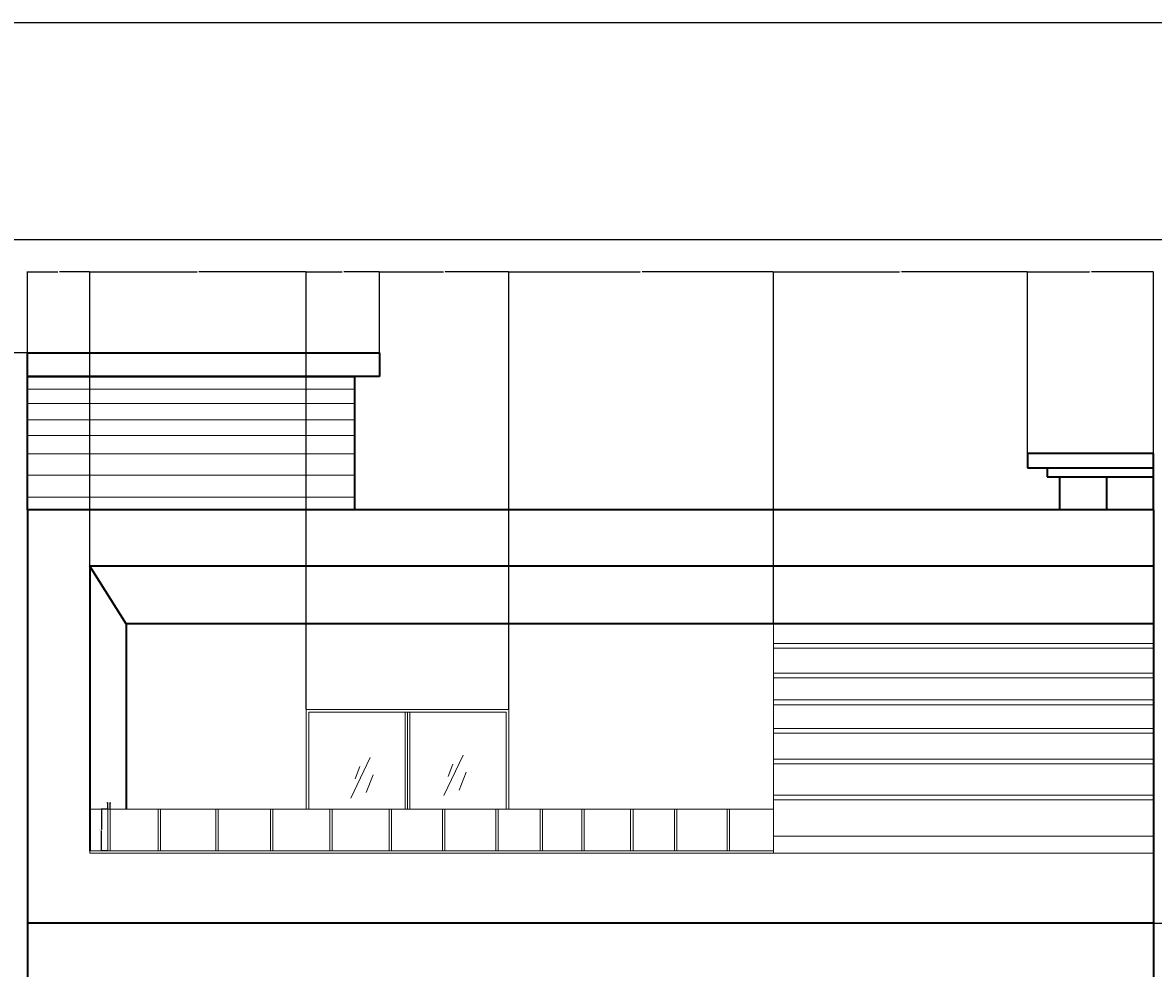
# Model space of a CAD drawing. Units: inches. Extents: x 1770 to 2988, y 1161 to 3221.
# Tile 36 of 44: x 2179 to 2655, y 2823 to 3221. Entities that reach past the tile are written whole.
import ezdxf

# ---------------------------------------------------------------- set-up
doc = ezdxf.new("R2010")
doc.units = ezdxf.units.IN
for name, color, linetype, lineweight in [('A-ANNO-DIMS', 2, 'Continuous', 18), ('A-ANNO-TTLB', 7, 'Continuous', 25), ('A-ELEV', 7, 'Continuous', 35), ('A-ELEV-DETL', 7, 'Continuous', 18), ('A-ELEV-GLAZ', 4, 'Continuous', 18)]:
    doc.layers.add(name, color=color, linetype=linetype, lineweight=lineweight)
doc.styles.get("Standard").update_dxf_attribs({"font": 'arial.ttf'})
doc.dimstyles.get("Standard").update_dxf_attribs({"dimtxt": 0.18, "dimasz": 0.18, "dimexe": 0.18, "dimexo": 0.0625, "dimgap": 0.09, "dimtad": 0, "dimtih": 1, "dimtoh": 1, "dimdec": 4, "dimzin": 0, "dimdsep": 46, "dimtxsty": 'Standard', "dimcen": 0.09, "dimadec": 0, "dimazin": 0, "dimtfac": 1, "dimtdec": 4, "dimtofl": 0, "dimtmove": 0, "dimatfit": 3, "dimfxl": 1, "dimtolj": 1, "dimtzin": 0, "dimarcsym": 0})

# ---------------------------------------------------------------- blocks, each defined once
blk = doc.blocks.new('GLASS-MARK-UPPER')
for p, q in [((8.2, 17.02), (0, 0)), ((3.76, 13.29), (1.82, 8.07)), ((9.37, 9.81), (6.4, 2.34))]:
    blk.add_line(p, q)
blk = doc.blocks.new('BALCONY-BALUSTER-ELEV')
for p, q in [((0, 17.5), (0, 0)), ((1, 0), (1, 17.5))]:
    blk.add_line(p, q)
blk = doc.blocks.new('*D54')
at = {"layer": 'A-ANNO-DIMS', "color": 0, "lineweight": -2, "transparency": 16777216}
for p, q in [((2215.14, 2890.3), (2212.39, 2890.3)), ((2212.57, 2890.12), (2212.57, 2881.73)), ((2212.57, 2872.97), (2212.57, 2881.36)), ((2215.14, 2872.79), (2212.39, 2872.79))]:
    blk.add_line(p, q, dxfattribs=at)
at = {"layer": 'A-ANNO-DIMS', "color": 0, "transparency": 16777216}
for points in [[(2212.54, 2890.12), (2212.6, 2890.12), (2212.57, 2890.3)], [(2212.54, 2872.97), (2212.6, 2872.97), (2212.57, 2872.79)]]:
    blk.add_solid(points, dxfattribs=at)
at = {"layer": 'Defpoints', "color": 0, "transparency": 16777216}
for p in [(2212.57, 2890.3), (2215.2, 2890.3), (2215.2, 2872.79)]:
    blk.add_point(p, dxfattribs=at)
at = {"layer": 'A-ANNO-DIMS', "color": 0, "transparency": 16777216, "insert": (2212.57, 2881.55), "char_height": 0.18, "attachment_point": 5}
blk.add_mtext('\\A1;BALUSTER 18 TYP.', dxfattribs=at)
blk = doc.blocks.new('*D55')
at = {"layer": 'A-ANNO-DIMS', "color": 0, "lineweight": -2, "transparency": 16777216}
for p, q in [((2215.02, 2892.92), (2214.84, 2892.92)), ((2215.2, 2890.36), (2215.2, 2893.1)), ((2216.2, 2890.36), (2216.2, 2893.1)), ((2216.38, 2892.92), (2216.56, 2892.92))]:
    blk.add_line(p, q, dxfattribs=at)
at = {"layer": 'A-ANNO-DIMS', "color": 0, "transparency": 16777216}
for points in [[(2215.02, 2892.95), (2215.02, 2892.89), (2215.2, 2892.92)], [(2216.38, 2892.95), (2216.38, 2892.89), (2216.2, 2892.92)]]:
    blk.add_solid(points, dxfattribs=at)
at = {"layer": 'Defpoints', "color": 0, "transparency": 16777216}
for p in [(2215.2, 2890.3), (2216.2, 2892.92), (2216.2, 2890.3)]:
    blk.add_point(p, dxfattribs=at)
at = {"layer": 'A-ANNO-DIMS', "color": 0, "transparency": 16777216, "insert": (2215.7, 2892.92), "char_height": 0.18, "attachment_point": 5}
blk.add_mtext('\\A1;1 TYP.', dxfattribs=at)
blk = doc.blocks.new('*D94')
at = {"layer": 'A-ANNO-DIMS', "color": 0, "lineweight": -2, "transparency": 16777216}
for p, q in [((2181.38, 3082.38), (2059.85, 3082.38)), ((2060.03, 3082.2), (2060.03, 2893.52)), ((2060.03, 2704.48), (2060.03, 2893.16)), ((2181.38, 2704.3), (2059.85, 2704.3))]:
    blk.add_line(p, q, dxfattribs=at)
at = {"layer": 'A-ANNO-DIMS', "color": 0, "transparency": 16777216}
for points in [[(2060, 3082.2), (2060.06, 3082.2), (2060.03, 3082.38)], [(2060, 2704.48), (2060.06, 2704.48), (2060.03, 2704.3)]]:
    blk.add_solid(points, dxfattribs=at)
at = {"layer": 'Defpoints', "color": 0, "transparency": 16777216}
for p in [(2060.03, 3082.38), (2181.44, 3082.38), (2181.44, 2704.3)]:
    blk.add_point(p, dxfattribs=at)
at = {"layer": 'A-ANNO-DIMS', "color": 0, "transparency": 16777216, "insert": (2060.03, 2893.34), "char_height": 0.18, "attachment_point": 5}
blk.add_mtext('\\A1;378.1', dxfattribs=at)
blk = doc.blocks.new('*D98')
at = {"layer": 'A-ANNO-DIMS', "color": 0, "lineweight": -2, "transparency": 16777216}
for p, q in [((2655.51, 2842.3), (2801.91, 2842.3)), ((2801.73, 2842.12), (2801.73, 2824.48)), ((2801.73, 2806.48), (2801.73, 2824.11)), ((2620.11, 2806.3), (2801.91, 2806.3))]:
    blk.add_line(p, q, dxfattribs=at)
at = {"layer": 'A-ANNO-DIMS', "color": 0, "transparency": 16777216}
for points in [[(2801.7, 2842.12), (2801.76, 2842.12), (2801.73, 2842.3)], [(2801.7, 2806.48), (2801.76, 2806.48), (2801.73, 2806.3)]]:
    blk.add_solid(points, dxfattribs=at)
at = {"layer": 'Defpoints', "color": 0, "transparency": 16777216}
for p in [(2655.44, 2842.3), (2801.73, 2842.3), (2620.05, 2806.3)]:
    blk.add_point(p, dxfattribs=at)
at = {"layer": 'A-ANNO-DIMS', "color": 0, "transparency": 16777216, "insert": (2801.73, 2824.3), "char_height": 0.18, "attachment_point": 5}
blk.add_mtext('\\A1;36', dxfattribs=at)
blk = doc.blocks.new('*D103')
at = {"layer": 'A-ANNO-DIMS', "color": 0, "lineweight": -2, "transparency": 16777216}
for p, q in [((2181.44, 3082.44), (2181.44, 3116.56)), ((2181.62, 3116.38), (2194.16, 3116.38)), ((2207.49, 3116.38), (2194.95, 3116.38)), ((2207.67, 2992.61), (2207.67, 3116.56))]:
    blk.add_line(p, q, dxfattribs=at)
at = {"layer": 'A-ANNO-DIMS', "color": 0, "transparency": 16777216}
for points in [[(2181.62, 3116.41), (2181.62, 3116.35), (2181.44, 3116.38)], [(2207.49, 3116.41), (2207.49, 3116.35), (2207.67, 3116.38)]]:
    blk.add_solid(points, dxfattribs=at)
at = {"layer": 'Defpoints', "color": 0, "transparency": 16777216}
for p in [(2207.67, 3116.38), (2181.44, 3082.38), (2207.67, 2992.55)]:
    blk.add_point(p, dxfattribs=at)
at = {"layer": 'A-ANNO-DIMS', "color": 0, "transparency": 16777216, "insert": (2194.56, 3116.38), "char_height": 0.18, "attachment_point": 5}
blk.add_mtext('\\A1;26.23', dxfattribs=at)
blk = doc.blocks.new('*D104')
at = {"layer": 'A-ANNO-DIMS', "color": 0, "lineweight": -2, "transparency": 16777216}
for p, q in [((2207.67, 2992.61), (2207.67, 3116.56)), ((2207.85, 3116.38), (2252.84, 3116.38)), ((2298.61, 3116.38), (2253.62, 3116.38)), ((2298.79, 2932.36), (2298.79, 3116.56))]:
    blk.add_line(p, q, dxfattribs=at)
at = {"layer": 'A-ANNO-DIMS', "color": 0, "transparency": 16777216}
for points in [[(2207.85, 3116.41), (2207.85, 3116.35), (2207.67, 3116.38)], [(2298.61, 3116.41), (2298.61, 3116.35), (2298.79, 3116.38)]]:
    blk.add_solid(points, dxfattribs=at)
at = {"layer": 'Defpoints', "color": 0, "transparency": 16777216}
for p in [(2298.79, 3116.38), (2207.67, 2992.55), (2298.79, 2932.3)]:
    blk.add_point(p, dxfattribs=at)
at = {"layer": 'A-ANNO-DIMS', "color": 0, "transparency": 16777216, "insert": (2253.23, 3116.38), "char_height": 0.18, "attachment_point": 5}
blk.add_mtext('\\A1;91.12', dxfattribs=at)
blk = doc.blocks.new('*D105')
at = {"layer": 'A-ANNO-DIMS', "color": 0, "lineweight": -2, "transparency": 16777216}
for p, q in [((2298.79, 2932.36), (2298.79, 3116.56)), ((2298.97, 3116.38), (2313.84, 3116.38)), ((2329.5, 3116.38), (2314.63, 3116.38)), ((2329.68, 3082.44), (2329.68, 3116.56))]:
    blk.add_line(p, q, dxfattribs=at)
at = {"layer": 'A-ANNO-DIMS', "color": 0, "transparency": 16777216}
for points in [[(2298.97, 3116.41), (2298.97, 3116.35), (2298.79, 3116.38)], [(2329.5, 3116.41), (2329.5, 3116.35), (2329.68, 3116.38)]]:
    blk.add_solid(points, dxfattribs=at)
at = {"layer": 'Defpoints', "color": 0, "transparency": 16777216}
for p in [(2329.68, 3116.38), (2329.68, 3082.38), (2298.79, 2932.3)]:
    blk.add_point(p, dxfattribs=at)
at = {"layer": 'A-ANNO-DIMS', "color": 0, "transparency": 16777216, "insert": (2314.23, 3116.38), "char_height": 0.18, "attachment_point": 5}
blk.add_mtext('\\A1;30.89', dxfattribs=at)
blk = doc.blocks.new('*D106')
at = {"layer": 'A-ANNO-DIMS', "color": 0, "lineweight": -2, "transparency": 16777216}
for p, q in [((2329.68, 3082.44), (2329.68, 3116.56)), ((2329.86, 3116.38), (2356.51, 3116.38)), ((2383.95, 3116.38), (2357.3, 3116.38)), ((2384.13, 2932.36), (2384.13, 3116.56))]:
    blk.add_line(p, q, dxfattribs=at)
at = {"layer": 'A-ANNO-DIMS', "color": 0, "transparency": 16777216}
for points in [[(2329.86, 3116.41), (2329.86, 3116.35), (2329.68, 3116.38)], [(2383.95, 3116.41), (2383.95, 3116.35), (2384.13, 3116.38)]]:
    blk.add_solid(points, dxfattribs=at)
at = {"layer": 'Defpoints', "color": 0, "transparency": 16777216}
for p in [(2384.13, 3116.38), (2329.68, 3082.38), (2384.13, 2932.3)]:
    blk.add_point(p, dxfattribs=at)
at = {"layer": 'A-ANNO-DIMS', "color": 0, "transparency": 16777216, "insert": (2356.91, 3116.38), "char_height": 0.18, "attachment_point": 5}
blk.add_mtext('\\A1;54.46', dxfattribs=at)
blk = doc.blocks.new('*D107')
at = {"layer": 'A-ANNO-DIMS', "color": 0, "lineweight": -2, "transparency": 16777216}
for p, q in [((2384.13, 2932.36), (2384.13, 3116.56)), ((2384.31, 3116.38), (2439.34, 3116.38)), ((2495.29, 3116.38), (2440.25, 3116.38)), ((2495.47, 2968.36), (2495.47, 3116.56))]:
    blk.add_line(p, q, dxfattribs=at)
at = {"layer": 'A-ANNO-DIMS', "color": 0, "transparency": 16777216}
for points in [[(2384.31, 3116.41), (2384.31, 3116.35), (2384.13, 3116.38)], [(2495.29, 3116.41), (2495.29, 3116.35), (2495.47, 3116.38)]]:
    blk.add_solid(points, dxfattribs=at)
at = {"layer": 'Defpoints', "color": 0, "transparency": 16777216}
for p in [(2495.47, 3116.38), (2495.47, 2968.3), (2384.13, 2932.3)]:
    blk.add_point(p, dxfattribs=at)
at = {"layer": 'A-ANNO-DIMS', "color": 0, "transparency": 16777216, "insert": (2439.8, 3116.38), "char_height": 0.18, "attachment_point": 5}
blk.add_mtext('\\A1;111.33', dxfattribs=at)
blk = doc.blocks.new('*D108')
at = {"layer": 'A-ANNO-DIMS', "color": 0, "lineweight": -2, "transparency": 16777216}
for p, q in [((2495.47, 2968.36), (2495.47, 3116.56)), ((2495.65, 3116.38), (2548.52, 3116.38)), ((2602.31, 3116.38), (2549.43, 3116.38)), ((2602.49, 3040.08), (2602.49, 3116.56))]:
    blk.add_line(p, q, dxfattribs=at)
at = {"layer": 'A-ANNO-DIMS', "color": 0, "transparency": 16777216}
for points in [[(2495.65, 3116.41), (2495.65, 3116.35), (2495.47, 3116.38)], [(2602.31, 3116.41), (2602.31, 3116.35), (2602.49, 3116.38)]]:
    blk.add_solid(points, dxfattribs=at)
at = {"layer": 'Defpoints', "color": 0, "transparency": 16777216}
for p in [(2602.49, 3116.38), (2602.49, 3040.02), (2495.47, 2968.3)]:
    blk.add_point(p, dxfattribs=at)
at = {"layer": 'A-ANNO-DIMS', "color": 0, "transparency": 16777216, "insert": (2548.98, 3116.38), "char_height": 0.18, "attachment_point": 5}
blk.add_mtext('\\A1;107.02', dxfattribs=at)
blk = doc.blocks.new('*D109')
at = {"layer": 'A-ANNO-DIMS', "color": 0, "lineweight": -2, "transparency": 16777216}
for p, q in [((2602.49, 3040.08), (2602.49, 3116.56)), ((2602.67, 3116.38), (2628.57, 3116.38)), ((2655.26, 3116.38), (2629.36, 3116.38)), ((2655.44, 3040.08), (2655.44, 3116.56))]:
    blk.add_line(p, q, dxfattribs=at)
at = {"layer": 'A-ANNO-DIMS', "color": 0, "transparency": 16777216}
for points in [[(2602.67, 3116.41), (2602.67, 3116.35), (2602.49, 3116.38)], [(2655.26, 3116.41), (2655.26, 3116.35), (2655.44, 3116.38)]]:
    blk.add_solid(points, dxfattribs=at)
at = {"layer": 'Defpoints', "color": 0, "transparency": 16777216}
for p in [(2655.44, 3116.38), (2602.49, 3040.02), (2655.44, 3040.02)]:
    blk.add_point(p, dxfattribs=at)
at = {"layer": 'A-ANNO-DIMS', "color": 0, "transparency": 16777216, "insert": (2628.96, 3116.38), "char_height": 0.18, "attachment_point": 5}
blk.add_mtext('\\A1;52.96', dxfattribs=at)

msp = doc.modelspace()

# ---------------------------------------------------------------- linework, layer by layer
at = {"layer": 'A-ANNO-TTLB'}
for points in [[(1769.9155, 3221.2788), (2987.7567, 3221.2788), (2987.7567, 1161.1516), (1769.9155, 1161.1516)], [(2073.6202, 3129.9468), (2769.3644, 3129.9468), (2769.3644, 2546.8952), (2073.6202, 2546.8952)]]:
    msp.add_lwpolyline(points, close=True, dxfattribs=at)
at = {"layer": 'A-ELEV'}
for p, q in [((2181.443, 3016.2969), (2181.443, 3082.3817)), ((2181.443, 3082.3817), (2329.6779, 3082.3817)), ((2329.6779, 3082.3817), (2329.6779, 3072.4167)), ((2329.6779, 3072.4167), (2181.443, 3072.4167)), ((2181.443, 3072.4167), (2319.1337, 3072.4167)), ((2319.1337, 3072.4167), (2319.1337, 3016.2969)), ((2655.443, 3040.0203), (2602.4869, 3040.0203)), ((2602.4869, 3040.0203), (2602.4869, 3033.8964)), ((2655.443, 3016.2969), (2655.443, 3040.0203)), ((2602.4869, 3033.8964), (2610.7495, 3033.8964)), ((2610.7495, 3033.8964), (2610.7495, 3030.156)), ((2610.7495, 3033.8964), (2655.443, 3033.8964)), ((2655.443, 3033.8964), (2655.443, 3033.8964)), ((2610.7495, 3030.156), (2615.954, 3030.156)), ((2615.954, 3030.156), (2615.954, 3016.2969)), ((2615.954, 3030.156), (2655.443, 3030.156)), ((2635.6985, 3030.156), (2635.6985, 3016.2969)), ((2181.443, 3016.2969), (2181.443, 2830.2969)), ((2655.443, 3016.2969), (2181.443, 3016.2969)), ((2655.443, 3016.2969), (2655.443, 2830.2969)), ((2655.443, 2992.5451), (2207.6717, 2992.5451)), ((2207.6717, 2992.5451), (2207.6717, 2872.7943)), ((2223.0291, 2968.2969), (2207.6717, 2992.5451)), ((2655.443, 2968.2969), (2223.0291, 2968.2969)), ((2223.0291, 2968.2969), (2223.0291, 2890.2969)), ((2181.443, 2890.2969), (2181.443, 2704.2969)), ((2655.443, 2890.2969), (2655.443, 2704.2969)), ((2655.443, 2842.2969), (2181.443, 2842.2969))]:
    msp.add_line(p, q, dxfattribs=at)
at = {"layer": 'A-ELEV-DETL'}
for p, q in [((2181.443, 3067.0892), (2319.1337, 3067.0892)), ((2181.443, 3061.03), (2319.1337, 3061.03)), ((2181.443, 3054.1618), (2319.1337, 3054.1618)), ((2181.443, 3047.5875), (2319.1337, 3047.5875)), ((2181.443, 3039.8117), (2319.1337, 3039.8117)), ((2181.443, 3030.8799), (2319.1337, 3030.8799)), ((2181.443, 3021.5728), (2319.1337, 3021.5728)), ((2495.4654, 2871.7943), (2495.4654, 2968.2969)), ((2495.4654, 2960.0436), (2655.443, 2960.0436)), ((2655.443, 2958.0436), (2495.4654, 2958.0436)), ((2655.443, 2960.0436), (2655.443, 2958.0436)), ((2495.4654, 2947.5038), (2655.443, 2947.5038)), ((2655.443, 2945.5038), (2495.4654, 2945.5038)), ((2495.4654, 2936.259), (2655.443, 2936.259)), ((2655.443, 2934.259), (2495.4654, 2934.259)), ((2495.4654, 2924.2391), (2655.443, 2924.2391)), ((2655.443, 2922.2391), (2495.4654, 2922.2391)), ((2495.4654, 2911.3321), (2655.443, 2911.3321)), ((2655.443, 2909.3321), (2495.4654, 2909.3321)), ((2495.4654, 2896.1676), (2655.443, 2896.1676)), ((2444.1544, 2890.2969), (2207.6717, 2890.2969)), ((2236.4714, 2890.2969), (2236.4714, 2872.7943)), ((2237.4714, 2872.7943), (2237.4714, 2890.2969)), ((2414.828, 2890.2969), (2414.828, 2872.7943)), ((2414.828, 2890.2969), (2414.828, 2872.7943)), ((2415.828, 2872.7943), (2415.828, 2890.2969)), ((2415.828, 2872.7943), (2415.828, 2890.2969)), ((2444.1544, 2890.2969), (2495.4654, 2890.2969)), ((2655.443, 2894.1676), (2495.4654, 2894.1676)), ((2655.443, 2872.7943), (2655.443, 2885.1589)), ((2655.443, 2878.9766), (2495.4654, 2878.9766)), ((2655.443, 2871.7943), (2655.443, 2878.9766)), ((2207.6717, 2872.7943), (2444.1544, 2872.7943)), ((2207.6717, 2872.7943), (2207.6717, 2871.7943)), ((2207.6717, 2871.7943), (2444.1544, 2871.7943)), ((2236.4714, 2872.7943), (2237.4714, 2872.7943)), ((2444.1544, 2872.7943), (2495.4654, 2872.7943)), ((2444.1544, 2871.7943), (2495.4654, 2871.7943)), ((2495.4654, 2871.7943), (2655.443, 2871.7943))]:
    msp.add_line(p, q, dxfattribs=at)
at = {"layer": 'A-ELEV-GLAZ'}
for p, q in [((2384.1342, 2932.2969), (2298.788, 2932.2969)), ((2298.788, 2932.2969), (2298.788, 2890.2969)), ((2340.4122, 2890.2969), (2340.4122, 2931.0547)), ((2341.46, 2931.0547), (2341.423, 2890.2969)), ((2341.46, 2931.0547), (2342.46, 2931.0547)), ((2342.46, 2931.0547), (2342.46, 2890.2969)), ((2384.1342, 2890.2969), (2384.1342, 2932.2969))]:
    msp.add_line(p, q, dxfattribs=at)
msp.add_lwpolyline([(2299.8748, 2890.2969), (2299.8748, 2931.0547), (2382.9497, 2931.0547), (2382.9497, 2890.2969)], dxfattribs=at)

# ---------------------------------------------------------------- block references
at = {"layer": 'A-ELEV-DETL'}
msp.add_blockref('BALCONY-BALUSTER-ELEV', (2215.2, 2872.794), dxfattribs=at)
at = {"layer": 'A-ELEV-DETL', "extrusion": (0, 0, -1), "zscale": -1, "rotation": 180}
for p in [(-2260.6562, 2890.2972), (-2283.7612, 2890.2972), (-2397.243, 2890.2972), (-2435.3651, 2890.2972), (-2475.9947, 2890.2972)]:
    msp.add_blockref('BALCONY-BALUSTER-ELEV', p, dxfattribs=at)
at = {"layer": 'A-ELEV-DETL', "rotation": 180}
for p in [(2309.6662, 2890.2972), (2334.6716, 2890.2972), (2357.1764, 2890.2972), (2379.5899, 2890.2972), (2454.8274, 2890.2972)]:
    msp.add_blockref('BALCONY-BALUSTER-ELEV', p, dxfattribs=at)
at = {"layer": 'A-ELEV-GLAZ'}
for p in [(2317.552, 2894.966), (2356.6975, 2895.9767)]:
    msp.add_blockref('GLASS-MARK-UPPER', p, dxfattribs=at)

# ---------------------------------------------------------------- dimensions: what is measured, and where the dimension line sits
at = {"layer": 'A-ANNO-DIMS'}
for base, p1, p2, picture, middle in [((2207.6717, 3116.3817), (2181.443, 3082.3817), (2207.6717, 2992.5451), '*D103', (2194.5573, 3116.3817)), ((2298.788, 3116.3817), (2207.6717, 2992.5451), (2298.788, 2932.2969), '*D104', (2253.2299, 3116.3817)), ((2329.6779, 3116.3817), (2298.788, 2932.2969), (2329.6779, 3082.3817), '*D105', (2314.233, 3116.3817)), ((2384.1342, 3116.3817), (2329.6779, 3082.3817), (2384.1342, 2932.2969), '*D106', (2356.906, 3116.3817)), ((2495.4654, 3116.3817), (2384.1342, 2932.2969), (2495.4654, 2968.2969), '*D107', (2439.7998, 3116.3817)), ((2602.4869, 3116.3817), (2495.4654, 2968.2969), (2602.4869, 3040.0203), '*D108', (2548.9761, 3116.3817)), ((2655.443, 3116.3817), (2602.4869, 3040.0203), (2655.443, 3040.0203), '*D109', (2628.9649, 3116.3817))]:
    dim = msp.add_linear_dim(base=base, p1=p1, p2=p2, dimstyle='Standard', override={"dimdec": 2, "dimlfac": 1, "dimrnd": 0, "dimzin": 0, "dimdsep": 46, "dimlunit": 2}, dxfattribs=at)
    dim.commit()
    dim.dimension.update_dxf_attribs({"geometry": picture, "text_midpoint": middle})
for base, p1, p2, override, picture, middle in [((2060.0309, 3082.3817), (2181.443, 2704.2969), (2181.443, 3082.3817), {"dimdec": 1, "dimlfac": 1, "dimrnd": 0, "dimzin": 0, "dimdsep": 46, "dimlunit": 2}, '*D94', (2060.0309, 2893.3393)), ((2801.7346, 2842.2969), (2620.0508, 2806.2969), (2655.443, 2842.2969), {"dimdec": 0, "dimlfac": 1, "dimrnd": 0, "dimzin": 0, "dimdsep": 46, "dimlunit": 2}, '*D98', (2801.7346, 2824.2969))]:
    dim = msp.add_linear_dim(base=base, p1=p1, p2=p2, angle=90, dimstyle='Standard', override=override, dxfattribs=at)
    dim.commit()
    dim.dimension.update_dxf_attribs({"geometry": picture, "text_midpoint": middle})
dim = msp.add_linear_dim(base=(2212.5745, 2890.2969), p1=(2215.1998, 2872.7943), p2=(2215.1998, 2890.2969), angle=90, text='BALUSTER <> TYP.', dimstyle='Standard', override={"dimdec": 0, "dimlfac": 1, "dimrnd": 0, "dimzin": 0, "dimdsep": 46, "dimlunit": 2}, dxfattribs=at)
dim.commit()
dim.dimension.update_dxf_attribs({"geometry": '*D54', "text_midpoint": (2212.5745, 2881.5456)})
dim = msp.add_linear_dim(base=(2216.1998, 2892.9223), p1=(2215.1998, 2890.2969), p2=(2216.1998, 2890.2969), text='<> TYP.', dimstyle='Standard', override={"dimdec": 0, "dimlfac": 1, "dimrnd": 0, "dimzin": 0, "dimdsep": 46, "dimlunit": 2}, dxfattribs=at)
dim.commit()
dim.dimension.update_dxf_attribs({"geometry": '*D55', "text_midpoint": (2215.6998, 2892.9223)})

doc.saveas('drawing.dxf')
